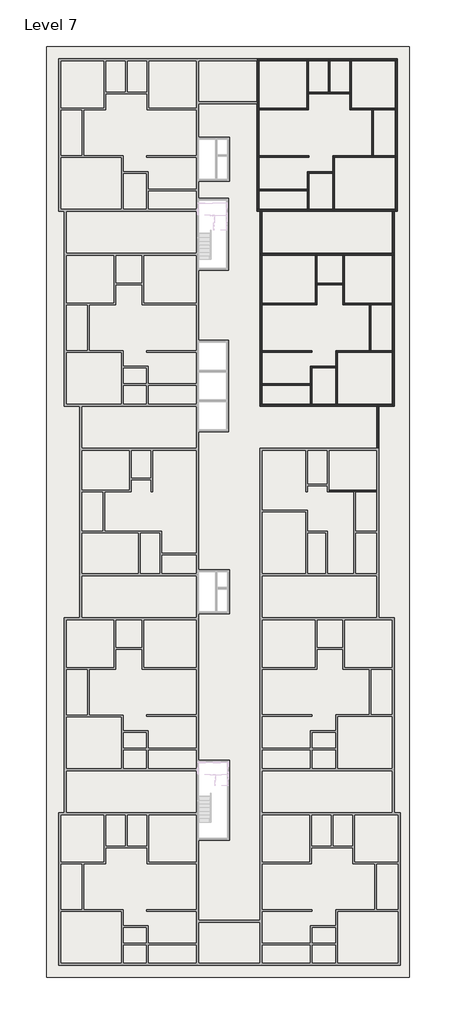
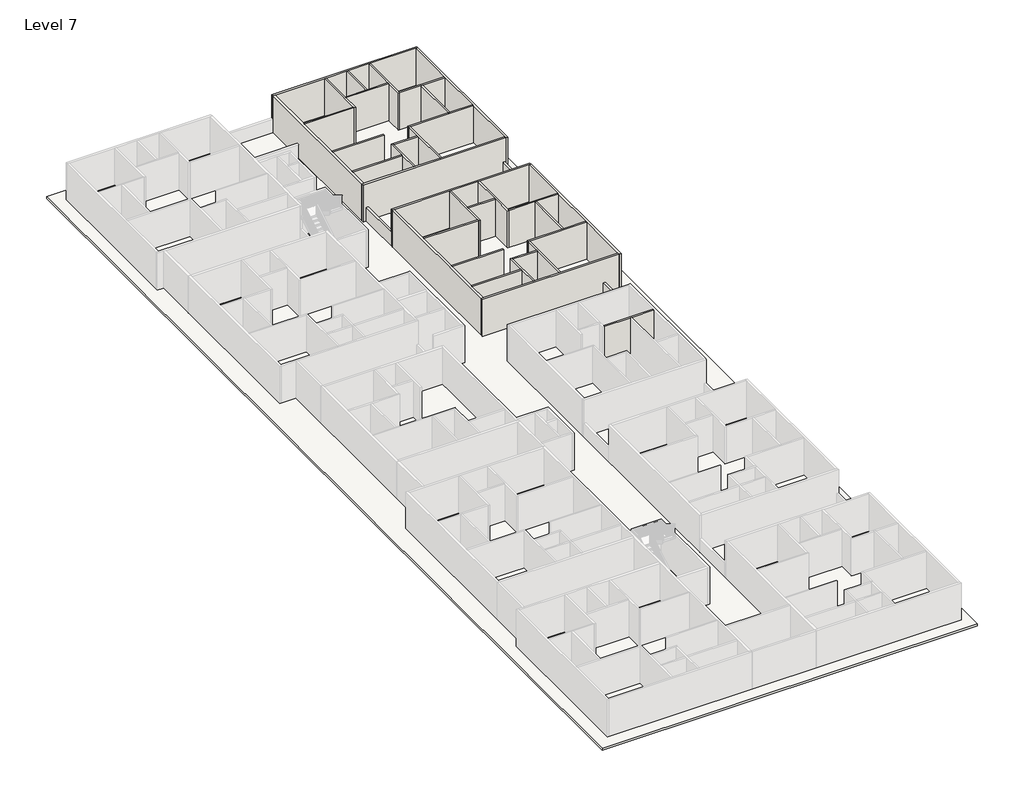
# One storey, part 4 of 8: 37 walls, 1 roof, 1 slab.
"""IFC4 building model written with IfcOpenShell, lengths in millimetres."""

from ifc_helpers import new_model, si_unit, frame, origin, place, context, project, spatial, polyline, outline, extrude, faceted_brep, element, save

model = new_model("IFC4")

# Units and contexts
model_context = context("Model", 3, world=origin())
ifc_project = project(units=[si_unit("LENGTHUNIT", "METRE", prefix="MILLI")], contexts=[model_context])

# Site, building, storey
site = spatial("IfcSite", under=ifc_project)
building = spatial("IfcBuilding", under=site)
storey = spatial("IfcBuildingStorey", under=building, Name="Level 7", Elevation=43522.6172466)

# Roof
placement = place(None, origin())
element("IfcRoof", 1, ObjectType="SLAB", at=placement, inside=storey, context=model_context, shape_type="SweptSolid", body=[
    extrude(outline(polyline([(-15237.9415084, -35021.5344126), (-15237.9415084, 36097.9216096), (12498.9443719, 36097.9216096), (12498.9443719, -35021.5344126), (-15237.9415084, -35021.5344126)]), holes=[polyline([(-3617.4415084, 29152.4900967), (-3617.4415084, 25799.6900967), (-1255.2415084, 25799.6900967), (-1255.2415084, 29152.4900967), (-3617.4415084, 29152.4900967)]), polyline([(-3617.4415084, 24490.1216096), (-3617.4415084, 19003.7216096), (-1331.4415084, 19003.7216096), (-1331.4415084, 24490.1216096), (-3617.4415084, 24490.1216096)]), polyline([(-3617.4415084, 13669.6303368), (-3617.4415084, 6659.2303368), (-1331.4415084, 6659.2303368), (-1331.4415084, 13669.6303368), (-3617.4415084, 13669.6303368)]), polyline([(-3617.4415084, -3882.2751812), (-3617.4415084, -7235.0751812), (-1255.2415084, -7235.0751812), (-1255.2415084, -3882.2751812), (-3617.4415084, -3882.2751812)]), polyline([(-3617.4415084, -18429.9851539), (-3617.4415084, -24525.9851539), (-1229.8415084, -24525.9851539), (-1229.8415084, -18429.9851539), (-3617.4415084, -18429.9851539)])]), frame((0.0, 0.0, 43522.6172466), z_axis=(0.0, 0.0, 1.0), x_axis=(1.0, 0.0, 0.0)), (0.0, 0.0, 1.0), 152.4),
])

# Slab
element("IfcSlab", 2, ObjectType="FLOOR", at=placement, inside=storey, context=model_context, shape_type="SweptSolid", body=[
    extrude(outline(polyline([(-14323.5415084, 35183.5216096), (11584.5443719, 35183.5216096), (11584.5443719, 23499.5216096), (11360.9214687, 23499.5216096), (11360.9214687, 8615.1216096), (10173.4714687, 8615.1216096), (10173.4714687, -7538.7344126), (11360.9214687, -7538.7344126), (11360.9214687, -22423.1344126), (11813.0584916, -22423.1344126), (11813.0584916, -34107.1344126), (11584.5443719, -34107.1344126), (-14323.5415084, -34107.1344126), (-14323.5415084, 35183.5216096)]), holes=[polyline([(-3617.4415084, 29152.4900967), (-3617.4415084, 25799.6900967), (-1255.2415084, 25799.6900967), (-1255.2415084, 29152.4900967), (-3617.4415084, 29152.4900967)]), polyline([(-3617.4415084, 24490.1216096), (-3617.4415084, 19003.7216096), (-1331.4415084, 19003.7216096), (-1331.4415084, 24490.1216096), (-3617.4415084, 24490.1216096)]), polyline([(-3617.4415084, 13669.6303368), (-3617.4415084, 6659.2303368), (-1331.4415084, 6659.2303368), (-1331.4415084, 13669.6303368), (-3617.4415084, 13669.6303368)]), polyline([(-3617.4415084, -3882.2751812), (-3617.4415084, -7235.0751812), (-1255.2415084, -7235.0751812), (-1255.2415084, -3882.2751812), (-3617.4415084, -3882.2751812)]), polyline([(-3617.4415084, -18429.9851539), (-3617.4415084, -24525.9851539), (-1229.8415084, -24525.9851539), (-1229.8415084, -18429.9851539), (-3617.4415084, -18429.9851539)])]), frame((0.0, 0.0, 42913.0172466), z_axis=(0.0, 0.0, 1.0), x_axis=(1.0, 0.0, 0.0)), (0.0, 0.0, 1.0), 609.6),
])

# Walls
element("IfcWall", 3, ObjectType="4.5\"", at=placement, inside=storey, context=model_context, shape_type="Brep", body=[
    faceted_brep([(6363.4714687, 2100.0216096, 43522.6172466), (8282.4584916, 2100.0216096, 43522.6172466), (8396.7584916, 2100.0216096, 43522.6172466), (10021.0714687, 2100.0216096, 43522.6172466), (10021.0714687, 2100.0216096, 46570.6172466), (8396.7584916, 2100.0216096, 46570.6172466), (8282.4584916, 2100.0216096, 46570.6172466), (6363.4714687, 2100.0216096, 46570.6172466), (6363.4714687, 2214.3216096, 43522.6172466), (6363.4714687, 2214.3216096, 46570.6172466), (10021.0714687, 2214.3216096, 46570.6172466), (10021.0714687, 2214.3216096, 43522.6172466)], [[[0, 1, 2, 3, 4, 5, 6, 7]], [[8, 9, 10, 11]], [[3, 2, 1, 0, 8, 11]], [[0, 7, 9, 8]], [[4, 3, 11, 10]], [[7, 6, 5, 4, 10, 9]]]),
])
element("IfcWall", 4, ObjectType="4.5\"", at=placement, inside=storey, context=model_context, shape_type="Brep", body=[
    faceted_brep([(5315.7214687, 20146.7216096, 43522.6172466), (5315.7214687, 16489.1216096, 43522.6172466), (5315.7214687, 16374.8216096, 43522.6172466), (5315.7214687, 16374.8216096, 46570.6172466), (5315.7214687, 16489.1216096, 46570.6172466), (5315.7214687, 20146.7216096, 46570.6172466), (5430.0214687, 20146.7216096, 43522.6172466), (5430.0214687, 20146.7216096, 46570.6172466), (5430.0214687, 18013.1216096, 46570.6172466), (5430.0214687, 17898.8216096, 46570.6172466), (5430.0214687, 16374.8216096, 46570.6172466), (5430.0214687, 16374.8216096, 43522.6172466), (5430.0214687, 17898.8216096, 43522.6172466), (5430.0214687, 18013.1216096, 43522.6172466)], [[[0, 1, 2, 3, 4, 5]], [[6, 7, 8, 9, 10, 11, 12, 13]], [[2, 1, 0, 6, 13, 12, 11]], [[0, 5, 7, 6]], [[3, 2, 11, 10]], [[5, 4, 3, 10, 9, 8, 7]]]),
])
element("IfcWall", 5, ObjectType="4.5\"", at=placement, inside=storey, context=model_context, shape_type="SweptSolid", body=[
    extrude(outline(polyline([(1259.3584916, 16489.1216096), (5315.7214687, 16489.1216096), (5315.7214687, 16374.8216096), (1259.3584916, 16374.8216096), (1259.3584916, 16489.1216096)])), frame((0.0, 0.0, 43522.6172466), z_axis=(0.0, 0.0, 1.0), x_axis=(1.0, 0.0, 0.0)), (0.0, 0.0, 1.0), 3048.0),
])
element("IfcWall", 6, ObjectType="4.5\"", at=placement, inside=storey, context=model_context, shape_type="SweptSolid", body=[
    extrude(outline(polyline([(7436.6214687, 17898.8216096), (5430.0214687, 17898.8216096), (5430.0214687, 18013.1216096), (7436.6214687, 18013.1216096), (7436.6214687, 17898.8216096)])), frame((0.0, 0.0, 43522.6172466), z_axis=(0.0, 0.0, 1.0), x_axis=(1.0, 0.0, 0.0)), (0.0, 0.0, 1.0), 3048.0),
])
element("IfcWall", 7, ObjectType="4.5\"", at=placement, inside=storey, context=model_context, shape_type="Brep", body=[
    faceted_brep([(7436.6214687, 20146.7216096, 43522.6172466), (7436.6214687, 18013.1216096, 43522.6172466), (7436.6214687, 17898.8216096, 43522.6172466), (7436.6214687, 16374.8216096, 43522.6172466), (7436.6214687, 16374.8216096, 46570.6172466), (7436.6214687, 17898.8216096, 46570.6172466), (7436.6214687, 18013.1216096, 46570.6172466), (7436.6214687, 20146.7216096, 46570.6172466), (7550.9214687, 20146.7216096, 43522.6172466), (7550.9214687, 20146.7216096, 46570.6172466), (7550.9214687, 16489.1216096, 46570.6172466), (7550.9214687, 16374.8216096, 46570.6172466), (7550.9214687, 16374.8216096, 43522.6172466), (7550.9214687, 16489.1216096, 43522.6172466)], [[[0, 1, 2, 3, 4, 5, 6, 7]], [[8, 9, 10, 11, 12, 13]], [[3, 2, 1, 0, 8, 13, 12]], [[0, 7, 9, 8]], [[4, 3, 12, 11]], [[7, 6, 5, 4, 11, 10, 9]]]),
])
element("IfcWall", 8, ObjectType="4.5\"", at=placement, inside=storey, context=model_context, shape_type="Brep", body=[
    faceted_brep([(7550.9214687, 16374.8216096, 43522.6172466), (9469.9084916, 16374.8216096, 43522.6172466), (9584.2084916, 16374.8216096, 43522.6172466), (11208.5214687, 16374.8216096, 43522.6172466), (11208.5214687, 16374.8216096, 46570.6172466), (9584.2084916, 16374.8216096, 46570.6172466), (9469.9084916, 16374.8216096, 46570.6172466), (7550.9214687, 16374.8216096, 46570.6172466), (7550.9214687, 16489.1216096, 43522.6172466), (7550.9214687, 16489.1216096, 46570.6172466), (11208.5214687, 16489.1216096, 46570.6172466), (11208.5214687, 16489.1216096, 43522.6172466)], [[[0, 1, 2, 3, 4, 5, 6, 7]], [[8, 9, 10, 11]], [[3, 2, 1, 0, 8, 11]], [[0, 7, 9, 8]], [[4, 3, 11, 10]], [[7, 6, 5, 4, 10, 9]]]),
])
element("IfcWall", 9, ObjectType="4.5\"", at=placement, inside=storey, context=model_context, shape_type="SweptSolid", body=[
    extrude(outline(polyline([(9469.9084916, 12869.6216096), (9469.9084916, 16374.8216096), (9584.2084916, 16374.8216096), (9584.2084916, 12869.6216096), (9469.9084916, 12869.6216096)])), frame((0.0, 0.0, 43522.6172466), z_axis=(0.0, 0.0, 1.0), x_axis=(1.0, 0.0, 0.0)), (0.0, 0.0, 1.0), 3048.0),
])
element("IfcWall", 10, ObjectType="4.5\"", at=placement, inside=storey, context=model_context, shape_type="Brep", body=[
    faceted_brep([(11208.5214687, 12869.6216096, 43522.6172466), (9584.2084916, 12869.6216096, 43522.6172466), (9469.9084916, 12869.6216096, 43522.6172466), (6885.4584916, 12869.6216096, 43522.6172466), (6885.4584916, 12869.6216096, 46570.6172466), (9469.9084916, 12869.6216096, 46570.6172466), (9584.2084916, 12869.6216096, 46570.6172466), (11208.5214687, 12869.6216096, 46570.6172466), (11208.5214687, 12755.3216096, 43522.6172466), (11208.5214687, 12755.3216096, 46570.6172466), (6999.7584916, 12755.3216096, 46570.6172466), (6885.4584916, 12755.3216096, 46570.6172466), (6885.4584916, 12755.3216096, 43522.6172466), (6999.7584916, 12755.3216096, 43522.6172466)], [[[0, 1, 2, 3, 4, 5, 6, 7]], [[8, 9, 10, 11, 12, 13]], [[3, 2, 1, 0, 8, 13, 12]], [[0, 7, 9, 8]], [[4, 3, 12, 11]], [[7, 6, 5, 4, 11, 10, 9]]]),
])
element("IfcWall", 11, ObjectType="4.5\"", at=placement, inside=storey, context=model_context, shape_type="Brep", body=[
    faceted_brep([(6885.4584916, 12755.3216096, 43522.6172466), (6885.4584916, 11663.1216096, 43522.6172466), (6885.4584916, 11548.8216096, 43522.6172466), (6885.4584916, 8767.5216096, 43522.6172466), (6885.4584916, 8767.5216096, 46570.6172466), (6885.4584916, 11548.8216096, 46570.6172466), (6885.4584916, 11663.1216096, 46570.6172466), (6885.4584916, 12755.3216096, 46570.6172466), (6999.7584916, 12755.3216096, 43522.6172466), (6999.7584916, 12755.3216096, 46570.6172466), (6999.7584916, 8767.5216096, 46570.6172466), (6999.7584916, 8767.5216096, 43522.6172466)], [[[0, 1, 2, 3, 4, 5, 6, 7]], [[8, 9, 10, 11]], [[3, 2, 1, 0, 8, 11]], [[0, 7, 9, 8]], [[4, 3, 11, 10]], [[7, 6, 5, 4, 10, 9]]]),
])
element("IfcWall", 12, ObjectType="4.5\"", at=placement, inside=storey, context=model_context, shape_type="Brep", body=[
    faceted_brep([(5056.6584916, 8767.5216096, 43522.6172466), (5056.6584916, 11548.8216096, 43522.6172466), (5056.6584916, 11663.1216096, 43522.6172466), (5056.6584916, 11663.1216096, 46570.6172466), (5056.6584916, 11548.8216096, 46570.6172466), (5056.6584916, 8767.5216096, 46570.6172466), (4942.3584916, 8767.5216096, 43522.6172466), (4942.3584916, 8767.5216096, 46570.6172466), (4942.3584916, 10215.3216096, 46570.6172466), (4942.3584916, 10329.6216096, 46570.6172466), (4942.3584916, 11663.1216096, 46570.6172466), (4942.3584916, 11663.1216096, 43522.6172466), (4942.3584916, 10329.6216096, 43522.6172466), (4942.3584916, 10215.3216096, 43522.6172466)], [[[0, 1, 2, 3, 4, 5]], [[6, 7, 8, 9, 10, 11, 12, 13]], [[2, 1, 0, 6, 13, 12, 11]], [[0, 5, 7, 6]], [[3, 2, 11, 10]], [[5, 4, 3, 10, 9, 8, 7]]]),
])
element("IfcWall", 13, ObjectType="4.5\"", at=placement, inside=storey, context=model_context, shape_type="SweptSolid", body=[
    extrude(outline(polyline([(6885.4584916, 11548.8216096), (5056.6584916, 11548.8216096), (5056.6584916, 11663.1216096), (6885.4584916, 11663.1216096), (6885.4584916, 11548.8216096)])), frame((0.0, 0.0, 43522.6172466), z_axis=(0.0, 0.0, 1.0), x_axis=(1.0, 0.0, 0.0)), (0.0, 0.0, 1.0), 3048.0),
])
element("IfcWall", 14, ObjectType="4.5\"", at=placement, inside=storey, context=model_context, shape_type="SweptSolid", body=[
    extrude(outline(polyline([(4942.3584916, 10215.3216096), (1259.3584916, 10215.3216096), (1259.3584916, 10329.6216096), (4942.3584916, 10329.6216096), (4942.3584916, 10215.3216096)])), frame((0.0, 0.0, 43522.6172466), z_axis=(0.0, 0.0, 1.0), x_axis=(1.0, 0.0, 0.0)), (0.0, 0.0, 1.0), 3048.0),
])
element("IfcWall", 15, ObjectType="4.5\"", at=placement, inside=storey, context=model_context, shape_type="SweptSolid", body=[
    extrude(outline(polyline([(5056.6584916, 12755.3216096), (1259.3584916, 12755.3216096), (1259.3584916, 12869.6216096), (5056.6584916, 12869.6216096), (5056.6584916, 12755.3216096)])), frame((0.0, 0.0, 43522.6172466), z_axis=(0.0, 0.0, 1.0), x_axis=(1.0, 0.0, 0.0)), (0.0, 0.0, 1.0), 3048.0),
])
element("IfcWall", 16, ObjectType="4.5\"", at=placement, inside=storey, context=model_context, shape_type="Brep", body=[
    faceted_brep([(4688.4443719, 35031.1216096, 43522.6172466), (4688.4443719, 31373.5216096, 43522.6172466), (4688.4443719, 31259.2216096, 43522.6172466), (4688.4443719, 31259.2216096, 46570.6172466), (4688.4443719, 31373.5216096, 46570.6172466), (4688.4443719, 35031.1216096, 46570.6172466), (4802.7443719, 35031.1216096, 43522.6172466), (4802.7443719, 35031.1216096, 46570.6172466), (4802.7443719, 32592.7216096, 46570.6172466), (4802.7443719, 32478.4216096, 46570.6172466), (4802.7443719, 31259.2216096, 46570.6172466), (4802.7443719, 31259.2216096, 43522.6172466), (4802.7443719, 32478.4216096, 43522.6172466), (4802.7443719, 32592.7216096, 43522.6172466)], [[[0, 1, 2, 3, 4, 5]], [[6, 7, 8, 9, 10, 11, 12, 13]], [[2, 1, 0, 6, 13, 12, 11]], [[0, 5, 7, 6]], [[3, 2, 11, 10]], [[5, 4, 3, 10, 9, 8, 7]]]),
])
element("IfcWall", 17, ObjectType="4.5\"", at=placement, inside=storey, context=model_context, shape_type="SweptSolid", body=[
    extrude(outline(polyline([(1030.8443719, 31373.5216096), (4688.4443719, 31373.5216096), (4688.4443719, 31259.2216096), (1030.8443719, 31259.2216096), (1030.8443719, 31373.5216096)])), frame((0.0, 0.0, 43522.6172466), z_axis=(0.0, 0.0, 1.0), x_axis=(1.0, 0.0, 0.0)), (0.0, 0.0, 1.0), 3048.0),
])
element("IfcWall", 18, ObjectType="4.5\"", at=placement, inside=storey, context=model_context, shape_type="Brep", body=[
    faceted_brep([(4802.7443719, 32478.4216096, 43522.6172466), (7965.0443719, 32478.4216096, 43522.6172466), (7965.0443719, 32478.4216096, 46570.6172466), (4802.7443719, 32478.4216096, 46570.6172466), (4802.7443719, 32592.7216096, 43522.6172466), (4802.7443719, 32592.7216096, 46570.6172466), (6326.7443719, 32592.7216096, 46570.6172466), (6441.0443719, 32592.7216096, 46570.6172466), (7965.0443719, 32592.7216096, 46570.6172466), (7965.0443719, 32592.7216096, 43522.6172466), (6441.0443719, 32592.7216096, 43522.6172466), (6326.7443719, 32592.7216096, 43522.6172466)], [[[0, 1, 2, 3]], [[4, 5, 6, 7, 8, 9, 10, 11]], [[1, 0, 4, 11, 10, 9]], [[0, 3, 5, 4]], [[2, 1, 9, 8]], [[3, 2, 8, 7, 6, 5]]]),
])
element("IfcWall", 19, ObjectType="4.5\"", at=placement, inside=storey, context=model_context, shape_type="SweptSolid", body=[
    extrude(outline(polyline([(6326.7443719, 32592.7216096), (6326.7443719, 35031.1216096), (6441.0443719, 35031.1216096), (6441.0443719, 32592.7216096), (6326.7443719, 32592.7216096)])), frame((0.0, 0.0, 43522.6172466), z_axis=(0.0, 0.0, 1.0), x_axis=(1.0, 0.0, 0.0)), (0.0, 0.0, 1.0), 3048.0),
])
element("IfcWall", 20, ObjectType="4.5\"", at=placement, inside=storey, context=model_context, shape_type="Brep", body=[
    faceted_brep([(7965.0443719, 35031.1216096, 43522.6172466), (7965.0443719, 32592.7216096, 43522.6172466), (7965.0443719, 32478.4216096, 43522.6172466), (7965.0443719, 31259.2216096, 43522.6172466), (7965.0443719, 31259.2216096, 46570.6172466), (7965.0443719, 32478.4216096, 46570.6172466), (7965.0443719, 32592.7216096, 46570.6172466), (7965.0443719, 35031.1216096, 46570.6172466), (8079.3443719, 35031.1216096, 43522.6172466), (8079.3443719, 35031.1216096, 46570.6172466), (8079.3443719, 31373.5216096, 46570.6172466), (8079.3443719, 31259.2216096, 46570.6172466), (8079.3443719, 31259.2216096, 43522.6172466), (8079.3443719, 31373.5216096, 43522.6172466)], [[[0, 1, 2, 3, 4, 5, 6, 7]], [[8, 9, 10, 11, 12, 13]], [[3, 2, 1, 0, 8, 13, 12]], [[0, 7, 9, 8]], [[4, 3, 12, 11]], [[7, 6, 5, 4, 11, 10, 9]]]),
])
element("IfcWall", 21, ObjectType="4.5\"", at=placement, inside=storey, context=model_context, shape_type="Brep", body=[
    faceted_brep([(8079.3443719, 31259.2216096, 43522.6172466), (9641.4443719, 31259.2216096, 43522.6172466), (9755.7443719, 31259.2216096, 43522.6172466), (11432.1443719, 31259.2216096, 43522.6172466), (11432.1443719, 31259.2216096, 46570.6172466), (9755.7443719, 31259.2216096, 46570.6172466), (9641.4443719, 31259.2216096, 46570.6172466), (8079.3443719, 31259.2216096, 46570.6172466), (8079.3443719, 31373.5216096, 43522.6172466), (8079.3443719, 31373.5216096, 46570.6172466), (11432.1443719, 31373.5216096, 46570.6172466), (11432.1443719, 31373.5216096, 43522.6172466)], [[[0, 1, 2, 3, 4, 5, 6, 7]], [[8, 9, 10, 11]], [[3, 2, 1, 0, 8, 11]], [[0, 7, 9, 8]], [[4, 3, 11, 10]], [[7, 6, 5, 4, 10, 9]]]),
])
element("IfcWall", 22, ObjectType="4.5\"", at=placement, inside=storey, context=model_context, shape_type="SweptSolid", body=[
    extrude(outline(polyline([(9641.4443719, 27754.0216096), (9641.4443719, 31259.2216096), (9755.7443719, 31259.2216096), (9755.7443719, 27754.0216096), (9641.4443719, 27754.0216096)])), frame((0.0, 0.0, 43522.6172466), z_axis=(0.0, 0.0, 1.0), x_axis=(1.0, 0.0, 0.0)), (0.0, 0.0, 1.0), 3048.0),
])
element("IfcWall", 23, ObjectType="4.5\"", at=placement, inside=storey, context=model_context, shape_type="Brep", body=[
    faceted_brep([(11432.1443719, 27754.0216096, 43522.6172466), (9755.7443719, 27754.0216096, 43522.6172466), (9641.4443719, 27754.0216096, 43522.6172466), (6656.9443719, 27754.0216096, 43522.6172466), (6656.9443719, 27754.0216096, 46570.6172466), (9641.4443719, 27754.0216096, 46570.6172466), (9755.7443719, 27754.0216096, 46570.6172466), (11432.1443719, 27754.0216096, 46570.6172466), (11432.1443719, 27639.7216096, 43522.6172466), (11432.1443719, 27639.7216096, 46570.6172466), (6771.2443719, 27639.7216096, 46570.6172466), (6656.9443719, 27639.7216096, 46570.6172466), (6656.9443719, 27639.7216096, 43522.6172466), (6771.2443719, 27639.7216096, 43522.6172466)], [[[0, 1, 2, 3, 4, 5, 6, 7]], [[8, 9, 10, 11, 12, 13]], [[3, 2, 1, 0, 8, 13, 12]], [[0, 7, 9, 8]], [[4, 3, 12, 11]], [[7, 6, 5, 4, 11, 10, 9]]]),
])
element("IfcWall", 24, ObjectType="4.5\"", at=placement, inside=storey, context=model_context, shape_type="Brep", body=[
    faceted_brep([(6656.9443719, 27639.7216096, 43522.6172466), (6656.9443719, 26547.5216096, 43522.6172466), (6656.9443719, 26433.2216096, 43522.6172466), (6656.9443719, 23651.9216096, 43522.6172466), (6656.9443719, 23651.9216096, 46570.6172466), (6656.9443719, 26433.2216096, 46570.6172466), (6656.9443719, 26547.5216096, 46570.6172466), (6656.9443719, 27639.7216096, 46570.6172466), (6771.2443719, 27639.7216096, 43522.6172466), (6771.2443719, 27639.7216096, 46570.6172466), (6771.2443719, 23651.9216096, 46570.6172466), (6771.2443719, 23651.9216096, 43522.6172466)], [[[0, 1, 2, 3, 4, 5, 6, 7]], [[8, 9, 10, 11]], [[3, 2, 1, 0, 8, 11]], [[0, 7, 9, 8]], [[4, 3, 11, 10]], [[7, 6, 5, 4, 10, 9]]]),
])
element("IfcWall", 25, ObjectType="4.5\"", at=placement, inside=storey, context=model_context, shape_type="SweptSolid", body=[
    extrude(outline(polyline([(4713.8443719, 25099.7216096), (1030.8443719, 25099.7216096), (1030.8443719, 25214.0216096), (4713.8443719, 25214.0216096), (4713.8443719, 25099.7216096)])), frame((0.0, 0.0, 43522.6172466), z_axis=(0.0, 0.0, 1.0), x_axis=(1.0, 0.0, 0.0)), (0.0, 0.0, 1.0), 3048.0),
])
element("IfcWall", 26, ObjectType="4.5\"", at=placement, inside=storey, context=model_context, shape_type="Brep", body=[
    faceted_brep([(4828.1443719, 23651.9216096, 43522.6172466), (4828.1443719, 26433.2216096, 43522.6172466), (4828.1443719, 26547.5216096, 43522.6172466), (4828.1443719, 26547.5216096, 46570.6172466), (4828.1443719, 26433.2216096, 46570.6172466), (4828.1443719, 23651.9216096, 46570.6172466), (4713.8443719, 23651.9216096, 43522.6172466), (4713.8443719, 23651.9216096, 46570.6172466), (4713.8443719, 25099.7216096, 46570.6172466), (4713.8443719, 25214.0216096, 46570.6172466), (4713.8443719, 26547.5216096, 46570.6172466), (4713.8443719, 26547.5216096, 43522.6172466), (4713.8443719, 25214.0216096, 43522.6172466), (4713.8443719, 25099.7216096, 43522.6172466)], [[[0, 1, 2, 3, 4, 5]], [[6, 7, 8, 9, 10, 11, 12, 13]], [[2, 1, 0, 6, 13, 12, 11]], [[0, 5, 7, 6]], [[3, 2, 11, 10]], [[5, 4, 3, 10, 9, 8, 7]]]),
])
element("IfcWall", 27, ObjectType="4.5\"", at=placement, inside=storey, context=model_context, shape_type="SweptSolid", body=[
    extrude(outline(polyline([(6656.9443719, 26433.2216096), (4828.1443719, 26433.2216096), (4828.1443719, 26547.5216096), (6656.9443719, 26547.5216096), (6656.9443719, 26433.2216096)])), frame((0.0, 0.0, 43522.6172466), z_axis=(0.0, 0.0, 1.0), x_axis=(1.0, 0.0, 0.0)), (0.0, 0.0, 1.0), 3048.0),
])
element("IfcWall", 28, ObjectType="4.5\"", at=placement, inside=storey, context=model_context, shape_type="SweptSolid", body=[
    extrude(outline(polyline([(4828.1443719, 27639.7216096), (1030.8443719, 27639.7216096), (1030.8443719, 27754.0216096), (4828.1443719, 27754.0216096), (4828.1443719, 27639.7216096)])), frame((0.0, 0.0, 43522.6172466), z_axis=(0.0, 0.0, 1.0), x_axis=(1.0, 0.0, 0.0)), (0.0, 0.0, 1.0), 3048.0),
])
element("IfcWall", 29, ObjectType="6\"", at=placement, inside=storey, context=model_context, shape_type="Brep", body=[
    faceted_brep([(1106.9584916, 20146.7216096, 46570.6172466), (1106.9584916, 20146.7216096, 43522.6172466), (1259.3584916, 20146.7216096, 43522.6172466), (5315.7214687, 20146.7216096, 43522.6172466), (5430.0214687, 20146.7216096, 43522.6172466), (7436.6214687, 20146.7216096, 43522.6172466), (7550.9214687, 20146.7216096, 43522.6172466), (11208.5214687, 20146.7216096, 43522.6172466), (11360.9214687, 20146.7216096, 43522.6172466), (11360.9214687, 20146.7216096, 46570.6172466), (11208.5214687, 20146.7216096, 46570.6172466), (7550.9214687, 20146.7216096, 46570.6172466), (7436.6214687, 20146.7216096, 46570.6172466), (5430.0214687, 20146.7216096, 46570.6172466), (5315.7214687, 20146.7216096, 46570.6172466), (1259.3584916, 20146.7216096, 46570.6172466), (1106.9584916, 20299.1216096, 43522.6172466), (1106.9584916, 20299.1216096, 44741.8172466), (1106.9584916, 20299.1216096, 46570.6172466), (11360.9214687, 20299.1216096, 46570.6172466), (11360.9214687, 20299.1216096, 44741.8172466), (11360.9214687, 20299.1216096, 43522.6172466), (11208.5214687, 20299.1216096, 43522.6172466), (1259.3584916, 20299.1216096, 43522.6172466)], [[[0, 1, 2, 3, 4, 5, 6, 7, 8, 9, 10, 11, 12, 13, 14, 15]], [[16, 17, 18, 19, 20, 21, 22, 23]], [[8, 7, 6, 5, 4, 3, 2, 1, 16, 23, 22, 21]], [[0, 18, 17, 16, 1]], [[8, 21, 20, 19, 9]], [[0, 15, 14, 13, 12, 11, 10, 9, 19, 18]]]),
])
element("IfcWall", 30, ObjectType="6\"", at=placement, inside=storey, context=model_context, shape_type="Brep", body=[
    faceted_brep([(11208.5214687, 20146.7216096, 46570.6172466), (11208.5214687, 20146.7216096, 43522.6172466), (11208.5214687, 16489.1216096, 43522.6172466), (11208.5214687, 16374.8216096, 43522.6172466), (11208.5214687, 12869.6216096, 43522.6172466), (11208.5214687, 12755.3216096, 43522.6172466), (11208.5214687, 8767.5216096, 43522.6172466), (11208.5214687, 8615.1216096, 43522.6172466), (11208.5214687, 8615.1216096, 46570.6172466), (11208.5214687, 8767.5216096, 46570.6172466), (11208.5214687, 12755.3216096, 46570.6172466), (11208.5214687, 12869.6216096, 46570.6172466), (11208.5214687, 16374.8216096, 46570.6172466), (11208.5214687, 16489.1216096, 46570.6172466), (11360.9214687, 20146.7216096, 43522.6172466), (11360.9214687, 20146.7216096, 46570.6172466), (11360.9214687, 8615.1216096, 46570.6172466), (11360.9214687, 8615.1216096, 43522.6172466)], [[[0, 1, 2, 3, 4, 5, 6, 7, 8, 9, 10, 11, 12, 13]], [[14, 15, 16, 17]], [[7, 6, 5, 4, 3, 2, 1, 14, 17]], [[8, 7, 17, 16]], [[0, 15, 14, 1]], [[0, 13, 12, 11, 10, 9, 8, 16, 15]]]),
])
element("IfcWall", 31, ObjectType="6\"", at=placement, inside=storey, context=model_context, shape_type="Brep", body=[
    faceted_brep([(11208.5214687, 8767.5216096, 43522.6172466), (6999.7584916, 8767.5216096, 43522.6172466), (6885.4584916, 8767.5216096, 43522.6172466), (5056.6584916, 8767.5216096, 43522.6172466), (4942.3584916, 8767.5216096, 43522.6172466), (1259.3584916, 8767.5216096, 43522.6172466), (1106.9584916, 8767.5216096, 43522.6172466), (1106.9584916, 8767.5216096, 46570.6172466), (1259.3584916, 8767.5216096, 46570.6172466), (4942.3584916, 8767.5216096, 46570.6172466), (5056.6584916, 8767.5216096, 46570.6172466), (6885.4584916, 8767.5216096, 46570.6172466), (6999.7584916, 8767.5216096, 46570.6172466), (11208.5214687, 8767.5216096, 46570.6172466), (11208.5214687, 8615.1216096, 43522.6172466), (11208.5214687, 8615.1216096, 46570.6172466), (1106.9584916, 8615.1216096, 46570.6172466), (1106.9584916, 8615.1216096, 43522.6172466), (10021.0714687, 8615.1216096, 43522.6172466), (10173.4714687, 8615.1216096, 43522.6172466)], [[[0, 1, 2, 3, 4, 5, 6, 7, 8, 9, 10, 11, 12, 13]], [[14, 15, 16, 17, 18, 19]], [[6, 5, 4, 3, 2, 1, 0, 14, 19, 18, 17]], [[0, 13, 15, 14]], [[7, 6, 17, 16]], [[13, 12, 11, 10, 9, 8, 7, 16, 15]]]),
])
element("IfcWall", 32, ObjectType="6\"", at=placement, inside=storey, context=model_context, shape_type="Brep", body=[
    faceted_brep([(1259.3584916, 8767.5216096, 43522.6172466), (1259.3584916, 10215.3216096, 43522.6172466), (1259.3584916, 10329.6216096, 43522.6172466), (1259.3584916, 12755.3216096, 43522.6172466), (1259.3584916, 12869.6216096, 43522.6172466), (1259.3584916, 16374.8216096, 43522.6172466), (1259.3584916, 16489.1216096, 43522.6172466), (1259.3584916, 20146.7216096, 43522.6172466), (1259.3584916, 20146.7216096, 46570.6172466), (1259.3584916, 16489.1216096, 46570.6172466), (1259.3584916, 16374.8216096, 46570.6172466), (1259.3584916, 12869.6216096, 46570.6172466), (1259.3584916, 12755.3216096, 46570.6172466), (1259.3584916, 10329.6216096, 46570.6172466), (1259.3584916, 10215.3216096, 46570.6172466), (1259.3584916, 8767.5216096, 46570.6172466), (1106.9584916, 8767.5216096, 43522.6172466), (1106.9584916, 8767.5216096, 46570.6172466), (1106.9584916, 20146.7216096, 46570.6172466), (1106.9584916, 20146.7216096, 43522.6172466)], [[[0, 1, 2, 3, 4, 5, 6, 7, 8, 9, 10, 11, 12, 13, 14, 15]], [[16, 17, 18, 19]], [[7, 6, 5, 4, 3, 2, 1, 0, 16, 19]], [[0, 15, 17, 16]], [[7, 19, 18, 8]], [[15, 14, 13, 12, 11, 10, 9, 8, 18, 17]]]),
])
element("IfcWall", 33, ObjectType="6\"", at=placement, inside=storey, context=model_context, shape_type="Brep", body=[
    faceted_brep([(878.4443719, 35031.1216096, 46570.6172466), (878.4443719, 35031.1216096, 43522.6172466), (1030.8443719, 35031.1216096, 43522.6172466), (4688.4443719, 35031.1216096, 43522.6172466), (4802.7443719, 35031.1216096, 43522.6172466), (6326.7443719, 35031.1216096, 43522.6172466), (6441.0443719, 35031.1216096, 43522.6172466), (7965.0443719, 35031.1216096, 43522.6172466), (8079.3443719, 35031.1216096, 43522.6172466), (11432.1443719, 35031.1216096, 43522.6172466), (11584.5443719, 35031.1216096, 43522.6172466), (11584.5443719, 35031.1216096, 46570.6172466), (11432.1443719, 35031.1216096, 46570.6172466), (8079.3443719, 35031.1216096, 46570.6172466), (7965.0443719, 35031.1216096, 46570.6172466), (6441.0443719, 35031.1216096, 46570.6172466), (6326.7443719, 35031.1216096, 46570.6172466), (4802.7443719, 35031.1216096, 46570.6172466), (4688.4443719, 35031.1216096, 46570.6172466), (1030.8443719, 35031.1216096, 46570.6172466), (878.4443719, 35183.5216096, 43522.6172466), (878.4443719, 35183.5216096, 46570.6172466), (11584.5443719, 35183.5216096, 46570.6172466), (11584.5443719, 35183.5216096, 43522.6172466)], [[[0, 1, 2, 3, 4, 5, 6, 7, 8, 9, 10, 11, 12, 13, 14, 15, 16, 17, 18, 19]], [[20, 21, 22, 23]], [[10, 9, 8, 7, 6, 5, 4, 3, 2, 1, 20, 23]], [[11, 10, 23, 22]], [[0, 21, 20, 1]], [[0, 19, 18, 17, 16, 15, 14, 13, 12, 11, 22, 21]]]),
])
element("IfcWall", 34, ObjectType="6\"", at=placement, inside=storey, context=model_context, shape_type="Brep", body=[
    faceted_brep([(11432.1443719, 35031.1216096, 43522.6172466), (11432.1443719, 31373.5216096, 43522.6172466), (11432.1443719, 31259.2216096, 43522.6172466), (11432.1443719, 27754.0216096, 43522.6172466), (11432.1443719, 27639.7216096, 43522.6172466), (11432.1443719, 23651.9216096, 43522.6172466), (11432.1443719, 23499.5216096, 43522.6172466), (11432.1443719, 23499.5216096, 46570.6172466), (11432.1443719, 23651.9216096, 46570.6172466), (11432.1443719, 27639.7216096, 46570.6172466), (11432.1443719, 27754.0216096, 46570.6172466), (11432.1443719, 31259.2216096, 46570.6172466), (11432.1443719, 31373.5216096, 46570.6172466), (11432.1443719, 35031.1216096, 46570.6172466), (11584.5443719, 35031.1216096, 43522.6172466), (11584.5443719, 35031.1216096, 46570.6172466), (11584.5443719, 23499.5216096, 46570.6172466), (11584.5443719, 23499.5216096, 43522.6172466)], [[[0, 1, 2, 3, 4, 5, 6, 7, 8, 9, 10, 11, 12, 13]], [[14, 15, 16, 17]], [[6, 5, 4, 3, 2, 1, 0, 14, 17]], [[0, 13, 15, 14]], [[7, 6, 17, 16]], [[13, 12, 11, 10, 9, 8, 7, 16, 15]]]),
])
element("IfcWall", 35, ObjectType="6\"", at=placement, inside=storey, context=model_context, shape_type="Brep", body=[
    faceted_brep([(11432.1443719, 23651.9216096, 43522.6172466), (6771.2443719, 23651.9216096, 43522.6172466), (6656.9443719, 23651.9216096, 43522.6172466), (4828.1443719, 23651.9216096, 43522.6172466), (4713.8443719, 23651.9216096, 43522.6172466), (1030.8443719, 23651.9216096, 43522.6172466), (878.4443719, 23651.9216096, 43522.6172466), (878.4443719, 23651.9216096, 46570.6172466), (1030.8443719, 23651.9216096, 46570.6172466), (4713.8443719, 23651.9216096, 46570.6172466), (4828.1443719, 23651.9216096, 46570.6172466), (6656.9443719, 23651.9216096, 46570.6172466), (6771.2443719, 23651.9216096, 46570.6172466), (11432.1443719, 23651.9216096, 46570.6172466), (11432.1443719, 23499.5216096, 43522.6172466), (11432.1443719, 23499.5216096, 46570.6172466), (878.4443719, 23499.5216096, 46570.6172466), (878.4443719, 23499.5216096, 43522.6172466), (1106.9584916, 23499.5216096, 43522.6172466), (1259.3584916, 23499.5216096, 43522.6172466), (11208.5214687, 23499.5216096, 43522.6172466), (11360.9214687, 23499.5216096, 43522.6172466)], [[[0, 1, 2, 3, 4, 5, 6, 7, 8, 9, 10, 11, 12, 13]], [[14, 15, 16, 17, 18, 19, 20, 21]], [[6, 5, 4, 3, 2, 1, 0, 14, 21, 20, 19, 18, 17]], [[0, 13, 15, 14]], [[7, 6, 17, 16]], [[13, 12, 11, 10, 9, 8, 7, 16, 15]]]),
])
element("IfcWall", 36, ObjectType="6\"", at=placement, inside=storey, context=model_context, shape_type="Brep", body=[
    faceted_brep([(1030.8443719, 23651.9216096, 43522.6172466), (1030.8443719, 25099.7216096, 43522.6172466), (1030.8443719, 25214.0216096, 43522.6172466), (1030.8443719, 27639.7216096, 43522.6172466), (1030.8443719, 27754.0216096, 43522.6172466), (1030.8443719, 31259.2216096, 43522.6172466), (1030.8443719, 31373.5216096, 43522.6172466), (1030.8443719, 35031.1216096, 43522.6172466), (1030.8443719, 35031.1216096, 46570.6172466), (1030.8443719, 31373.5216096, 46570.6172466), (1030.8443719, 31259.2216096, 46570.6172466), (1030.8443719, 27754.0216096, 46570.6172466), (1030.8443719, 27639.7216096, 46570.6172466), (1030.8443719, 25214.0216096, 46570.6172466), (1030.8443719, 25099.7216096, 46570.6172466), (1030.8443719, 23651.9216096, 46570.6172466), (878.4443719, 23651.9216096, 43522.6172466), (878.4443719, 23651.9216096, 46570.6172466), (878.4443719, 35031.1216096, 46570.6172466), (878.4443719, 35031.1216096, 43522.6172466), (878.4443719, 31897.3197155, 43522.6172466), (878.4443719, 31744.9197155, 43522.6172466)], [[[0, 1, 2, 3, 4, 5, 6, 7, 8, 9, 10, 11, 12, 13, 14, 15]], [[16, 17, 18, 19, 20, 21]], [[7, 6, 5, 4, 3, 2, 1, 0, 16, 21, 20, 19]], [[0, 15, 17, 16]], [[7, 19, 18, 8]], [[15, 14, 13, 12, 11, 10, 9, 8, 18, 17]]]),
])
element("IfcWall", 37, ObjectType="6\" 2", at=placement, inside=storey, context=model_context, shape_type="SweptSolid", body=[
    extrude(outline(polyline([(1106.9584916, 20299.1216096), (1106.9584916, 23499.5216096), (1259.3584916, 23499.5216096), (1259.3584916, 20299.1216096), (1106.9584916, 20299.1216096)])), frame((0.0, 0.0, 43522.6172466), z_axis=(0.0, 0.0, 1.0), x_axis=(1.0, 0.0, 0.0)), (0.0, 0.0, 1.0), 1219.2),
])
element("IfcWall", 38, ObjectType="6\" 2", at=placement, inside=storey, context=model_context, shape_type="SweptSolid", body=[
    extrude(outline(polyline([(11208.5214687, 20299.1216096), (11208.5214687, 23499.5216096), (11360.9214687, 23499.5216096), (11360.9214687, 20299.1216096), (11208.5214687, 20299.1216096)])), frame((0.0, 0.0, 43522.6172466), z_axis=(0.0, 0.0, 1.0), x_axis=(1.0, 0.0, 0.0)), (0.0, 0.0, 1.0), 1219.2),
])
element("IfcWall", 39, ObjectType="6\" 2", at=placement, inside=storey, context=model_context, shape_type="SweptSolid", body=[
    extrude(outline(polyline([(10021.0714687, 5414.7216096), (10021.0714687, 8615.1216096), (10173.4714687, 8615.1216096), (10173.4714687, 5414.7216096), (10021.0714687, 5414.7216096)])), frame((0.0, 0.0, 43522.6172466), z_axis=(0.0, 0.0, 1.0), x_axis=(1.0, 0.0, 0.0)), (0.0, 0.0, 1.0), 1219.2),
])

save(model, "model.ifc")

# Revit data of these elements
# Type "SLAB"
#   Assembly Code = "B1020"
#   Layers, outside or top first: 0' - 6" "Damp-proofing" (function 1)
# Type "FLOOR"
#   Assembly Code = "B1010"
#   Function = 0
#   Layers, outside or top first: 2' - 0" "Tile, Porcelain, 4in" (function 1)
# Type "4.5\""
#   Assembly Code = "B2010"
#   Layers, outside or top first: 0' - 4 1/2" "WALLS" (function 1)
# Type "6\""
#   Assembly Code = "B2010"
#   Layers, outside or top first: 0' - 6" "WALLS" (function 1)
# Type "6\" 2"
#   Assembly Code = "B2010"
#   Layers, outside or top first: 0' - 6" "4'" (function 1)
# Element 1 (IfcRoof, "SLAB")
#   built-in parameter 1001705 = 143.291 (stored number, unit not read)
#   built-in parameter 1001710 = 33615
#   Phase Created = New Construction
#   Materials on its faces: "Damp-proofing"
# Element 2 (IfcSlab, "FLOOR")
#   built-in parameter 1001955 = 3.14159 (stored number, unit not read)
#   Height Offset From Level = 0' - 0"
#   Phase Created = New Construction
#   Materials on its faces: "Tile, Porcelain, 4in"
# Elements 3, 4, 5, 6, 7, 8, 9, 10, 11, 12, 13, 14, 15, 16, 17, 18, 19, 20, 21, 22, 23, 24, 25, 26, 27, 28 (IfcWall, "4.5\"")
#   Top Offset = 0' - 0"
#   Base Offset = 0' - 0"
#   Unconnected Height = 10' - 0"
#   wall height = 10' - 0"
#   Phase Created = New Construction
#   Base Constraint = Level 7
#   Materials on its faces: "WALLS"
# Elements 29, 30, 31, 32, 33, 34, 35, 36 (IfcWall, "6\"")
#   Top Offset = 0' - 0"
#   Base Offset = 0' - 0"
#   Unconnected Height = 10' - 0"
#   wall height = 10' - 0"
#   Phase Created = New Construction
#   Base Constraint = Level 7
#   Materials on its faces: "WALLS"
# Elements 37, 38, 39 (IfcWall, "6\" 2")
#   Top Offset = 0' - 0"
#   Base Offset = 0' - 0"
#   Unconnected Height = 4' - 0"
#   wall height = 4' - 0"
#   Phase Created = New Construction
#   Base Constraint = Level 7
#   Materials on its faces: "4'"
# Materials
#   "Damp-proofing": class "Generic", colour RGB 127 127 127, transparency 0, Description = "Damp-proofing", Cost = 0
#   "Tile, Porcelain, 4in": class "Generic", colour RGB 89 87 158, transparency 0, Description = "Porcelain tile, 4\", white", Cost = 0
#   "WALLS": class "Generic", colour RGB 120 120 120, transparency 0, Cost = 0
#   "4'": class "Generic", colour RGB 120 120 120, transparency 0, Cost = 0
